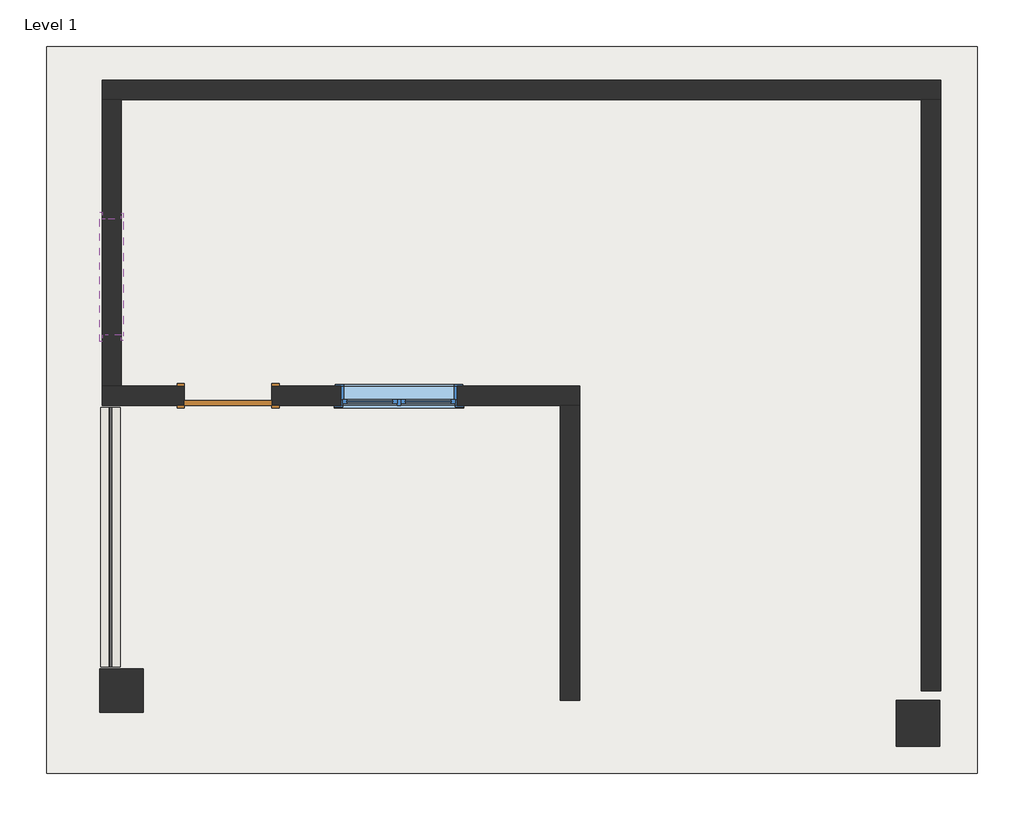
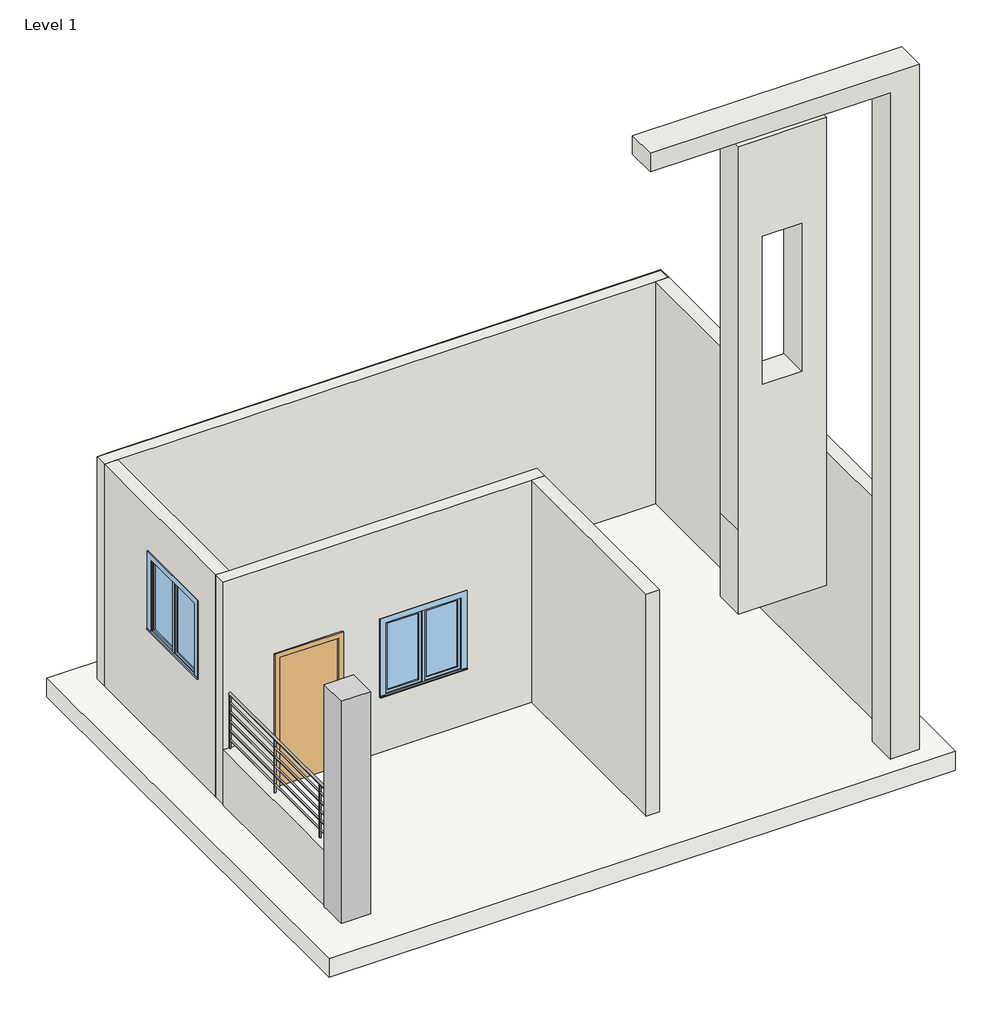
# One storey: 7 walls, 2 windows, 1 column, 1 door, 1 railing, 1 slab.
"""IFC4 building model written with IfcOpenShell, lengths in millimetres."""

from ifc_helpers import new_model, si_unit, point, frame, frame_2d, origin, origin_with_axes, place, context, project, spatial, polyline, circle_curve, trimmed, segment, composite_curve, outline, extrude, faceted_brep, transform, mapped, element, save
from components import column_ce396696, door_54dd4da4, walls_1_walls_1_cb3e8ea8, window_0862ab64

model = new_model("IFC4")

# Units and contexts
model_context = context("Model", 3, world=origin())
ifc_project = project(units=[si_unit("LENGTHUNIT", "METRE", prefix="MILLI")], contexts=[model_context])

# Site, building, storey
site = spatial("IfcSite", under=ifc_project)
building = spatial("IfcBuilding", under=site)
storey = spatial("IfcBuildingStorey", under=building, Name="Level 1", Elevation=0.0)

# Column
placement = place(None, origin())
column_shape = column_ce396696(model_context)
element("IfcColumn", 1, ObjectType="Rectangular Column : 18\" x 18\"", at=placement, inside=storey, context=model_context, shape_type="MappedRepresentation", body=[
    mapped(column_shape, transform((-11365.149546, 5994.8170892, 0.0), x_axis=(1.0, 0.0, 0.0), y_axis=(0.0, 1.0, 0.0), z_axis=(0.0, 0.0, 1.0))),
])

# Door
door_shape = door_54dd4da4(model_context)
element("IfcDoor", 2, ObjectType="Single-Flush : 36\" x 84\"", at=placement, inside=storey, context=model_context, shape_type="MappedRepresentation", body=[
    mapped(door_shape, transform((-10247.549546, 9086.334124, 0.0), x_axis=(-1.0, 0.0, 0.0), y_axis=(0.0, -1.0, 0.0), z_axis=(0.0, 0.0, 1.0))),
])

# Railing
element("IfcRailing", 3, ObjectType="Handrail - Pipe", at=placement, inside=storey, context=model_context, shape_type="SweptSolid", body=[
    extrude(outline(composite_curve([segment(trimmed(circle_curve(frame_2d((1809.75, -11479.449546)), 19.05), [point((1809.75, -11498.499546))], [point((1809.75, -11460.399546))], False, "CARTESIAN"), True, "CONTINUOUS"), segment(trimmed(circle_curve(frame_2d((1809.75, -11479.449546)), 19.05), [point((1809.75, -11460.399546))], [point((1809.75, -11498.499546))], False, "CARTESIAN"), True, "CONTINUOUS")], self_intersect=False)), frame((0.0, 6247.884124, 0.0), z_axis=(0.0, 1.0, 0.0), x_axis=(0.0, 0.0, 1.0)), (0.0, 0.0, 1.0), 2717.8),
    extrude(outline(composite_curve([segment(trimmed(circle_curve(frame_2d((1663.7, -11479.449546)), 12.7), [point((1663.7, -11466.749546))], [point((1663.7, -11492.149546))], False, "CARTESIAN"), True, "CONTINUOUS"), segment(trimmed(circle_curve(frame_2d((1663.7, -11479.449546)), 12.7), [point((1663.7, -11492.149546))], [point((1663.7, -11466.749546))], False, "CARTESIAN"), True, "CONTINUOUS")], self_intersect=False)), frame((0.0, 6247.884124, 0.0), z_axis=(0.0, 1.0, 0.0), x_axis=(0.0, 0.0, 1.0)), (0.0, 0.0, 1.0), 2717.8),
    extrude(outline(composite_curve([segment(trimmed(circle_curve(frame_2d((1511.3, -11479.449546)), 12.7), [point((1511.3, -11466.749546))], [point((1511.3, -11492.149546))], False, "CARTESIAN"), True, "CONTINUOUS"), segment(trimmed(circle_curve(frame_2d((1511.3, -11479.449546)), 12.7), [point((1511.3, -11492.149546))], [point((1511.3, -11466.749546))], False, "CARTESIAN"), True, "CONTINUOUS")], self_intersect=False)), frame((0.0, 6247.884124, 0.0), z_axis=(0.0, 1.0, 0.0), x_axis=(0.0, 0.0, 1.0)), (0.0, 0.0, 1.0), 2717.8),
    extrude(outline(composite_curve([segment(trimmed(circle_curve(frame_2d((1358.9, -11479.449546)), 12.7), [point((1358.9, -11466.749546))], [point((1358.9, -11492.149546))], False, "CARTESIAN"), True, "CONTINUOUS"), segment(trimmed(circle_curve(frame_2d((1358.9, -11479.449546)), 12.7), [point((1358.9, -11492.149546))], [point((1358.9, -11466.749546))], False, "CARTESIAN"), True, "CONTINUOUS")], self_intersect=False)), frame((0.0, 6247.884124, 0.0), z_axis=(0.0, 1.0, 0.0), x_axis=(0.0, 0.0, 1.0)), (0.0, 0.0, 1.0), 2717.8),
    extrude(outline(composite_curve([segment(trimmed(circle_curve(frame_2d((1206.5, -11479.449546)), 12.7), [point((1206.5, -11466.749546))], [point((1206.5, -11492.149546))], False, "CARTESIAN"), True, "CONTINUOUS"), segment(trimmed(circle_curve(frame_2d((1206.5, -11479.449546)), 12.7), [point((1206.5, -11492.149546))], [point((1206.5, -11466.749546))], False, "CARTESIAN"), True, "CONTINUOUS")], self_intersect=False)), frame((0.0, 6247.884124, 0.0), z_axis=(0.0, 1.0, 0.0), x_axis=(0.0, 0.0, 1.0)), (0.0, 0.0, 1.0), 2717.8),
    extrude(outline(composite_curve([segment(trimmed(circle_curve(frame_2d((1054.1, -11479.449546)), 12.7), [point((1054.1, -11466.749546))], [point((1054.1, -11492.149546))], False, "CARTESIAN"), True, "CONTINUOUS"), segment(trimmed(circle_curve(frame_2d((1054.1, -11479.449546)), 12.7), [point((1054.1, -11492.149546))], [point((1054.1, -11466.749546))], False, "CARTESIAN"), True, "CONTINUOUS")], self_intersect=False)), frame((0.0, 6247.884124, 0.0), z_axis=(0.0, 1.0, 0.0), x_axis=(0.0, 0.0, 1.0)), (0.0, 0.0, 1.0), 2717.8),
    extrude(outline(composite_curve([segment(trimmed(circle_curve(frame_2d((-11479.449546, 6527.284124)), 12.7), [point((-11466.749546, 6527.284124))], [point((-11492.149546, 6527.284124))], False, "CARTESIAN"), True, "CONTINUOUS"), segment(trimmed(circle_curve(frame_2d((-11479.449546, 6527.284124)), 12.7), [point((-11492.149546, 6527.284124))], [point((-11466.749546, 6527.284124))], False, "CARTESIAN"), True, "CONTINUOUS")], self_intersect=False)), frame((0.0, 0.0, 914.4), z_axis=(0.0, 0.0, 1.0), x_axis=(1.0, 0.0, 0.0)), (0.0, 0.0, 1.0), 876.3),
    extrude(outline(composite_curve([segment(trimmed(circle_curve(frame_2d((-11479.449546, 7746.484124)), 12.7), [point((-11466.749546, 7746.484124))], [point((-11492.149546, 7746.484124))], False, "CARTESIAN"), True, "CONTINUOUS"), segment(trimmed(circle_curve(frame_2d((-11479.449546, 7746.484124)), 12.7), [point((-11492.149546, 7746.484124))], [point((-11466.749546, 7746.484124))], False, "CARTESIAN"), True, "CONTINUOUS")], self_intersect=False)), frame((0.0, 0.0, 914.4), z_axis=(0.0, 0.0, 1.0), x_axis=(1.0, 0.0, 0.0)), (0.0, 0.0, 1.0), 876.3),
    extrude(outline(composite_curve([segment(trimmed(circle_curve(frame_2d((-11479.449546, 6260.584124)), 12.7), [point((-11466.749546, 6260.584124))], [point((-11492.149546, 6260.584124))], False, "CARTESIAN"), True, "CONTINUOUS"), segment(trimmed(circle_curve(frame_2d((-11479.449546, 6260.584124)), 12.7), [point((-11492.149546, 6260.584124))], [point((-11466.749546, 6260.584124))], False, "CARTESIAN"), True, "CONTINUOUS")], self_intersect=False)), frame((0.0, 0.0, 914.4), z_axis=(0.0, 0.0, 1.0), x_axis=(1.0, 0.0, 0.0)), (0.0, 0.0, 1.0), 876.3),
    extrude(outline(composite_curve([segment(trimmed(circle_curve(frame_2d((-11479.449546, 8952.984124)), 12.7), [point((-11466.749546, 8952.984124))], [point((-11492.149546, 8952.984124))], False, "CARTESIAN"), True, "CONTINUOUS"), segment(trimmed(circle_curve(frame_2d((-11479.449546, 8952.984124)), 12.7), [point((-11492.149546, 8952.984124))], [point((-11466.749546, 8952.984124))], False, "CARTESIAN"), True, "CONTINUOUS")], self_intersect=False)), frame((0.0, 0.0, 914.4), z_axis=(0.0, 0.0, 1.0), x_axis=(1.0, 0.0, 0.0)), (0.0, 0.0, 1.0), 876.3),
])

# Slab
element("IfcSlab", 4, ObjectType="Generic - 12\"", at=placement, inside=storey, context=model_context, shape_type="SweptSolid", body=[
    extrude(outline(polyline([(-2396.4681702, 12748.9793041), (-2396.4681702, 5128.9793041), (-12150.0681702, 5128.9793041), (-12150.0681702, 12748.9793041), (-2396.4681702, 12748.9793041)])), frame((0.0, 0.0, -304.8), z_axis=(0.0, 0.0, 1.0), x_axis=(1.0, 0.0, 0.0)), (0.0, 0.0, 1.0), 304.8),
])

# Walls
element("IfcWall", 5, ObjectType="Generic - 8\"", at=placement, inside=storey, context=model_context, shape_type="Brep", body=[
    faceted_brep([(-11568.349546, 12192.4170892, 0.0), (-11365.149546, 12192.4170892, 0.0), (-2983.149546, 12192.4170892, 0.0), (-2779.949546, 12192.4170892, 0.0), (-2779.949546, 12192.4170892, 3657.6), (-2789.0236868, 12192.4170892, 3657.6), (-2983.149546, 12192.4170892, 3657.6), (-11365.149546, 12192.4170892, 3657.6), (-11390.549546, 12192.4170892, 3657.6), (-11568.349546, 12192.4170892, 3657.6), (-11568.349546, 12395.6170892, 0.0), (-11568.349546, 12395.6170892, 3657.6), (-11390.549546, 12395.6170892, 3657.6), (-2789.0236868, 12395.6170892, 3657.6), (-2779.949546, 12395.6170892, 3657.6), (-2779.949546, 12395.6170892, 0.0), (-11568.349546, 12388.334124, 3657.6), (-2779.949546, 12388.334124, 3657.6), (-2789.0236868, 12388.334124, 3657.6)], [[[0, 1, 2, 3, 4, 5, 6, 7, 8, 9]], [[10, 11, 12, 13, 14, 15]], [[3, 2, 1, 0, 10, 15]], [[0, 9, 16, 11, 10]], [[4, 3, 15, 14, 17]], [[5, 4, 17, 18]], [[13, 12, 11, 16, 18]], [[17, 14, 13, 18]], [[9, 8, 7, 6, 5, 18, 16]]]),
])
element("IfcWall", 6, ObjectType="Generic - 8\"", at=placement, inside=storey, context=model_context, shape_type="SweptSolid", body=[
    extrude(outline(polyline([(9187.934124, 0.0), (9187.934124, 3657.6), (12192.4170892, 3657.6), (12192.4170892, 0.0), (9187.934124, 0.0)]), holes=[polyline([(10944.1756066, 2878.4838915), (9724.9756066, 2878.4838915), (9724.9756066, 1659.2838915), (10944.1756066, 1659.2838915), (10944.1756066, 2878.4838915)])]), frame((-11568.349546, 0.0, 0.0), z_axis=(1.0, 0.0, 0.0), x_axis=(0.0, 1.0, 0.0)), (0.0, 0.0, 1.0), 203.2),
])
element("IfcWall", 7, ObjectType="Generic - 8\"", at=placement, inside=storey, context=model_context, shape_type="SweptSolid", body=[
    extrude(outline(polyline([(-2983.149546, 5994.8170892), (-2983.149546, 12192.4170892), (-2779.949546, 12192.4170892), (-2779.949546, 5994.8170892), (-2983.149546, 5994.8170892)])), origin_with_axes(), (0.0, 0.0, 1.0), 3657.6),
])
element("IfcWall", 8, ObjectType="Generic - 8\"", at=placement, inside=storey, context=model_context, shape_type="Brep", body=[
    faceted_brep([(-11568.349546, 8984.734124, 0.0), (-10704.749546, 8984.734124, 0.0), (-10704.749546, 8984.734124, 2133.6), (-9790.349546, 8984.734124, 2133.6), (-9790.349546, 8984.734124, 0.0), (-6767.749546, 8984.734124, 0.0), (-6564.549546, 8984.734124, 0.0), (-6564.549546, 8984.734124, 3657.6), (-6767.749546, 8984.734124, 3657.6), (-11568.349546, 8984.734124, 3657.6), (-9066.449546, 8984.734124, 2133.6), (-7847.249546, 8984.734124, 2133.6), (-7847.249546, 8984.734124, 914.4), (-9066.449546, 8984.734124, 914.4), (-10704.749546, 9187.934124, 2133.6), (-10704.749546, 9187.934124, 0.0), (-11365.149546, 9187.934124, 0.0), (-11568.349546, 9187.934124, 0.0), (-11568.349546, 9187.934124, 3657.6), (-11365.149546, 9187.934124, 3657.6), (-6564.549546, 9187.934124, 3657.6), (-6564.549546, 9187.934124, 0.0), (-9790.349546, 9187.934124, 0.0), (-9790.349546, 9187.934124, 2133.6), (-9066.449546, 9187.934124, 2133.6), (-9066.449546, 9187.934124, 914.4), (-7847.249546, 9187.934124, 914.4), (-7847.249546, 9187.934124, 2133.6)], [[[0, 1, 2, 3, 4, 5, 6, 7, 8, 9], [10, 11, 12, 13]], [[14, 15, 16, 17, 18, 19, 20, 21, 22, 23], [24, 25, 26, 27]], [[22, 21, 6, 5, 4]], [[17, 16, 15, 1, 0]], [[9, 8, 7, 20, 19, 18]], [[7, 6, 21, 20]], [[0, 9, 18, 17]], [[2, 1, 15, 14]], [[3, 2, 14, 23]], [[4, 3, 23, 22]], [[25, 24, 10, 13]], [[26, 25, 13, 12]], [[27, 26, 12, 11]], [[24, 27, 11, 10]]]),
])
element("IfcWall", 9, ObjectType="Generic - 8\"", at=placement, inside=storey, context=model_context, shape_type="SweptSolid", body=[
    extrude(outline(polyline([(-6767.749546, 5893.2170892), (-6767.749546, 8984.734124), (-6564.549546, 8984.734124), (-6564.549546, 5893.2170892), (-6767.749546, 5893.2170892)])), origin_with_axes(), (0.0, 0.0, 1.0), 3657.6),
])
element("IfcWall", 10, ObjectType="Generic - 8\"", at=placement, inside=storey, context=model_context, shape_type="SweptSolid", body=[
    extrude(outline(polyline([(-11581.049546, 6247.884124), (-11581.049546, 8965.684124), (-11377.849546, 8965.684124), (-11377.849546, 6247.884124), (-11581.049546, 6247.884124)])), origin_with_axes(), (0.0, 0.0, 1.0), 914.4),
])
walls_1_walls_1_shape = walls_1_walls_1_cb3e8ea8(model_context)
element("IfcWall", 11, ObjectType="Walls 1 : Walls 1", at=placement, inside=storey, context=model_context, shape_type="MappedRepresentation", body=[
    mapped(walls_1_walls_1_shape, transform((0.0, 0.0, 0.0), x_axis=(1.0, 0.0, 0.0), y_axis=(0.0, 1.0, 0.0), z_axis=(0.0, 0.0, 1.0))),
])

# Windows
window_shape = window_0862ab64(model_context)
element("IfcWindow", 12, ObjectType="Casement Dbl with Trim : 48\" x 48\"", at=placement, inside=storey, context=model_context, shape_type="MappedRepresentation", body=[
    mapped(window_shape, transform((-8456.849546, 9105.384124, 0.0), x_axis=(-1.0, 0.0, 0.0), y_axis=(0.0, -1.0, 0.0), z_axis=(0.0, 0.0, 1.0))),
])
element("IfcWindow", 13, ObjectType="Casement Dbl with Trim : 48\" x 48\"", at=placement, inside=storey, context=model_context, shape_type="MappedRepresentation", body=[
    mapped(window_shape, transform((-11447.699546, 10334.5756066, 744.8838915), x_axis=(0.0, 1.0, 0.0), y_axis=(-1.0, 0.0, 0.0), z_axis=(0.0, 0.0, 1.0))),
])

save(model, "model.ifc")

# Revit data of these elements
# Type "Rectangular Column : 18\" x 18\""
#   Assembly Code = "B1010200"
#   Depth = 1' - 6"
#   Offset Base = 0' - 0"
#   Offset Top = 0' - 0"
#   Width = 1' - 6"
#   Material = none
# Type "Single-Flush : 36\" x 84\""
#   Type Mark = "1"
#   Construction Type Id = "MDOOR"
#   Assembly Code = "C1020"
#   Analytic Construction = "Metal"
#   Thickness = 0' - 2"
#   Heat Transfer Coefficient (U) = 0.651978 BTU/(h·ft²·°F)
#   Height = 7' - 0"
#   Trim Projection Ext = 0' - 1"
#   Trim Projection Int = 0' - 1"
#   Trim Width = 0' - 3"
#   Width = 3' - 0"
#   Define Thermal Properties by = 1
#   Door Material = Door - Panel
#   Frame Material = Door - Frame
#   Visual Light Transmittance = 0
#   Solar Heat Gain Coefficient = 0
#   Function = (empty or 0)
#   Wall Closure = (empty or 0)
# Type "Handrail - Pipe"
#   Assembly Code = "C2010400"
#   built-in parameter 1008612 = 0.0416667 (stored number, unit not read)
#   built-in parameter 1008611 = 0.0833333 (stored number, unit not read)
#   built-in parameter 1008609 = 4 (stored number, unit not read)
#   built-in parameter 1008604 = 0.166667 (stored number, unit not read)
#   built-in parameter 1008603 = 0.166667 (stored number, unit not read)
#   Railing Height = 3' - 0"
#   built-in parameter 1008630 = 2
#   built-in parameter 1008610 = 1
#   built-in parameter 1008605 = 1
#   built-in parameter 1008618 = Baluster - Round : 1"
# Type "Generic - 12\""
#   Assembly Code = "B1010"
#   Function = 0
#   Layers, outside or top first: 1' - 0" no material (function 1)
# Type "Generic - 8\""
#   Assembly Code = "B2010"
#   Layers, outside or top first: 0' - 8" no material (function 1)
# Type "Casement Dbl with Trim : 48\" x 48\""
#   Type Mark = "10"
#   Construction Type Id = "GSP4R"
#   Assembly Code = "B2020100"
#   Analytic Construction = "1/8 in Pilkington single glazing"
#   Visual Light Transmittance = 0.9
#   Thermal Resistance (R) = 1.53941 (h·ft²·°F)/BTU
#   Solar Heat Gain Coefficient = 0.78
#   Heat Transfer Coefficient (U) = 0.6496 BTU/(h·ft²·°F)
#   Height = 4' - 0"
#   Default Sill Height = 3' - 0"
#   Trim Projection - Ext. = 0' - 0 1/2"
#   Trim Projection - Int. = 0' - 0 3/4"
#   Trim Width - Exterior = 0' - 3 1/2"
#   Trim Width - Interior = 0' - 3 1/2"
#   Width = 4' - 0"
#   Window Inset = 0' - 0 3/4"
#   Define Thermal Properties by = 1
#   Glass Pane Material = Glass
#   Sash Material = Sash
#   Trim Exterior Material = Trim
#   Trim Interior Material = Trim
#   Wall Closure = (empty or 0)
# Element 1 (IfcColumn, "Rectangular Column : 18\" x 18\"")
#   Phase Created = New Construction
# Element 2 (IfcDoor, "Single-Flush : 36\" x 84\"")
#   Phase Created = New Construction
#   Materials on its faces: "Door - Frame", "Door - Panel"
# Element 3 (IfcRailing, "Handrail - Pipe")
#   built-in parameter 1008621 = 3 (stored number, unit not read)
#   Phase Created = New Construction
# Element 4 (IfcSlab, "Generic - 12\"")
#   Height Offset From Level = 0' - 0"
#   Phase Created = New Construction
#   Materials on its faces: "Default Floor"
# Elements 5, 6, 7, 8, 9 (IfcWall, "Generic - 8\"")
#   Top Offset = 0' - 0"
#   Base Offset = 0' - 0"
#   Unconnected Height = 12' - 0"
#   wall height = 12' - 0"
#   Phase Created = New Construction
#   Base Constraint = Level 1
#   Materials on its faces: "Default Wall"
# Element 10 (IfcWall, "Generic - 8\"")
#   Top Offset = 0' - 0"
#   Base Offset = 0' - 0"
#   Unconnected Height = 3' - 0"
#   wall height = 3' - 0"
#   Phase Created = New Construction
#   Base Constraint = Level 1
#   Materials on its faces: "Default Wall"
# Element 11 (IfcWall, "Walls 1 : Walls 1")
#   Phase Created = New Construction
#   Materials on its faces: "Default Wall"
# Element 12 (IfcWindow, "Casement Dbl with Trim : 48\" x 48\"")
#   Mark = "2"
#   Phase Created = New Construction
#   Materials on its faces: "Sash", "Trim", "Glass"
# Element 13 (IfcWindow, "Casement Dbl with Trim : 48\" x 48\"")
#   Mark = "4"
#   Phase Created = New Construction
#   Materials on its faces: "Sash", "Trim", "Glass"
# Materials
#   "Door - Panel": class "Wood", colour RGB 210 159 95, transparency 0
#   "Door - Frame": colour RGB 118 70 51, transparency 0
#   "Glass": class "Glass", colour RGB 0 128 192, transparency 0.75, Description = "Soda Lime Glass", Cost = 0
#   "Sash": class "Wood", colour RGB 224 178 126, transparency 0
#   "Trim": class "Wood", colour RGB 224 178 126, transparency 0
#   "Default Floor": colour RGB 128 128 128, transparency 0
#   "Default Wall": colour RGB 128 128 128, transparency 0
